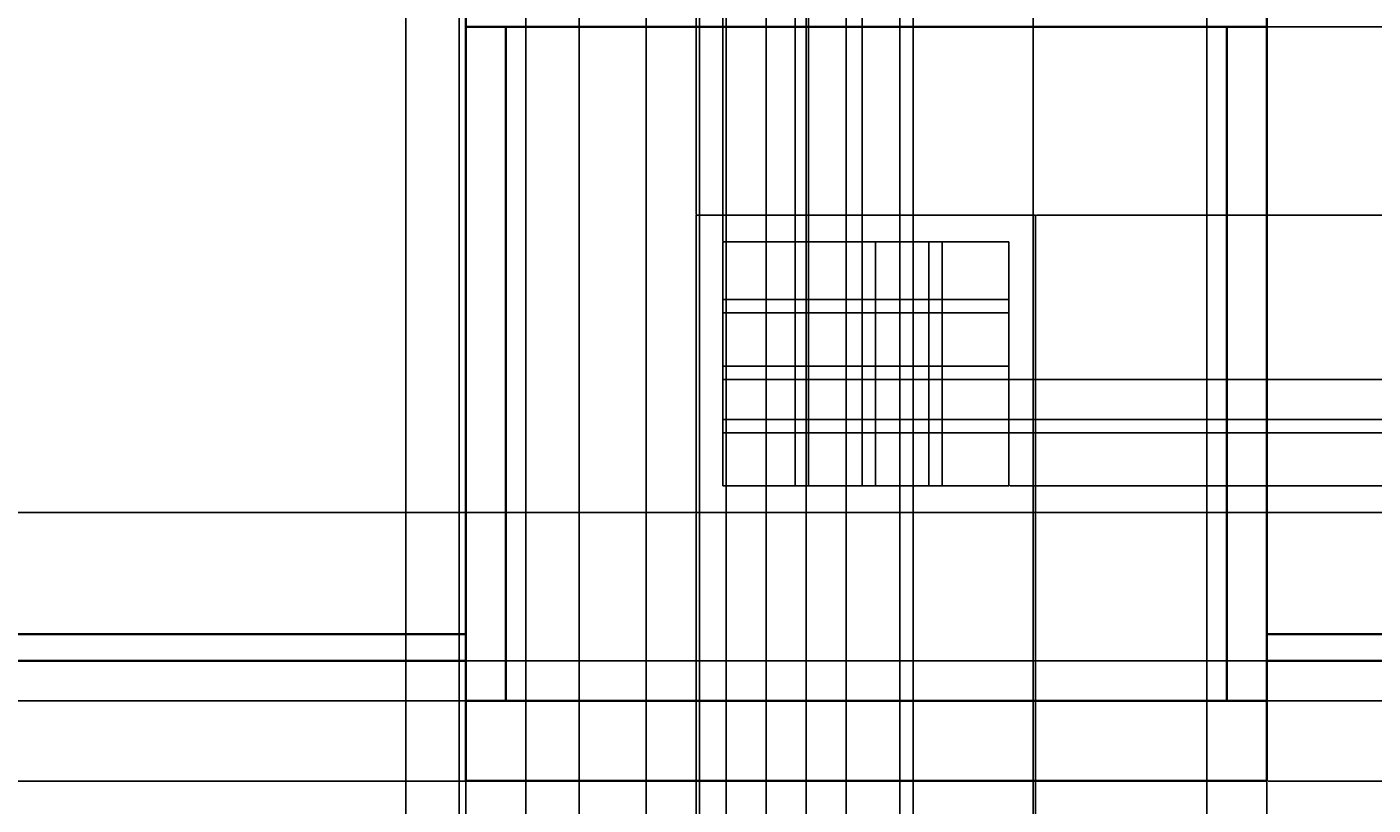
# Model space of a CAD drawing. Units: inches. Extents: x 2154 to 2740, y 571 to 1084.
# Tile 10 of 13: x 2384 to 2485, y 969 to 1027. Entities that reach past the tile are written whole.
import ezdxf

# ---------------------------------------------------------------- set-up
doc = ezdxf.new("R2010")
doc.units = ezdxf.units.IN
for name, color, linetype, lineweight in [('A-ANNO-DIMS', 2, 'Continuous', 18), ('A-GLAZ', 4, 'Continuous', 25), ('A-ROOF', 1, 'Continuous', 35)]:
    doc.layers.add(name, color=color, linetype=linetype, lineweight=lineweight)
doc.styles.get("Standard").update_dxf_attribs({"font": 'arial.ttf'})
doc.dimstyles.get("Standard").update_dxf_attribs({"dimtxt": 0.18, "dimasz": 0.18, "dimexe": 0.18, "dimexo": 0.0625, "dimgap": 0.09, "dimtad": 0, "dimtih": 1, "dimtoh": 1, "dimdec": 4, "dimzin": 0, "dimdsep": 46, "dimtxsty": 'Standard', "dimcen": 0.09, "dimadec": 0, "dimazin": 0, "dimtfac": 1, "dimtdec": 4, "dimtofl": 0, "dimtmove": 0, "dimatfit": 3, "dimfxl": 1, "dimtolj": 1, "dimtzin": 0, "dimarcsym": 0})

# ---------------------------------------------------------------- blocks, each defined once
blk = doc.blocks.new('*D7')
at = {"layer": 'A-ANNO-DIMS', "color": 0, "lineweight": -2, "transparency": 16777216}
for p, q in [((2181.21, 981.59), (2181.21, 1084.04)), ((2181.39, 1083.86), (2446.92, 1083.86)), ((2713.03, 1083.86), (2447.49, 1083.86)), ((2713.21, 981.59), (2713.21, 1084.04))]:
    blk.add_line(p, q, dxfattribs=at)
at = {"layer": 'A-ANNO-DIMS', "color": 0, "transparency": 16777216}
for points in [[(2181.39, 1083.89), (2181.39, 1083.83), (2181.21, 1083.86)], [(2713.03, 1083.89), (2713.03, 1083.83), (2713.21, 1083.86)]]:
    blk.add_solid(points, dxfattribs=at)
at = {"layer": 'Defpoints', "color": 0, "transparency": 16777216}
for p in [(2713.21, 1083.86), (2181.21, 981.53), (2713.21, 981.53)]:
    blk.add_point(p, dxfattribs=at)
at = {"layer": 'A-ANNO-DIMS', "color": 0, "transparency": 16777216, "insert": (2447.21, 1083.86), "char_height": 0.18, "attachment_point": 5}
blk.add_mtext('\\A1;532', dxfattribs=at)
blk = doc.blocks.new('*D9')
at = {"layer": 'A-ANNO-DIMS', "color": 0, "lineweight": -2, "transparency": 16777216}
for p, q in [((2417.21, 970.47), (2417.21, 570.5)), ((2477.21, 970.47), (2477.21, 570.5)), ((2417.39, 570.68), (2446.99, 570.68)), ((2477.03, 570.68), (2447.43, 570.68))]:
    blk.add_line(p, q, dxfattribs=at)
at = {"layer": 'A-ANNO-DIMS', "color": 0, "transparency": 16777216}
for points in [[(2417.39, 570.71), (2417.39, 570.65), (2417.21, 570.68)], [(2477.03, 570.71), (2477.03, 570.65), (2477.21, 570.68)]]:
    blk.add_solid(points, dxfattribs=at)
at = {"layer": 'Defpoints', "color": 0, "transparency": 16777216}
for p in [(2417.21, 970.53), (2477.21, 970.53), (2477.21, 570.68)]:
    blk.add_point(p, dxfattribs=at)
at = {"layer": 'A-ANNO-DIMS', "color": 0, "transparency": 16777216, "insert": (2447.21, 570.68), "char_height": 0.18, "attachment_point": 5}
blk.add_mtext('\\A1;60', dxfattribs=at)
blk = doc.blocks.new('*D10')
at = {"layer": 'A-ANNO-DIMS', "color": 0, "lineweight": -2, "transparency": 16777216}
for p, q in [((2447.14, 1057.01), (2154.18, 1057.01)), ((2154.36, 1056.83), (2154.36, 827.45)), ((2154.36, 597.71), (2154.36, 827.09)), ((2181.14, 597.53), (2154.18, 597.53))]:
    blk.add_line(p, q, dxfattribs=at)
at = {"layer": 'A-ANNO-DIMS', "color": 0, "transparency": 16777216}
for points in [[(2154.33, 1056.83), (2154.39, 1056.83), (2154.36, 1057.01)], [(2154.33, 597.71), (2154.39, 597.71), (2154.36, 597.53)]]:
    blk.add_solid(points, dxfattribs=at)
at = {"layer": 'Defpoints', "color": 0, "transparency": 16777216}
for p in [(2154.36, 1057.01), (2447.21, 1057.01), (2181.21, 597.53)]:
    blk.add_point(p, dxfattribs=at)
at = {"layer": 'A-ANNO-DIMS', "color": 0, "transparency": 16777216, "insert": (2154.36, 827.27), "char_height": 0.18, "attachment_point": 5}
blk.add_mtext('\\A1;459.5', dxfattribs=at)
blk = doc.blocks.new('*D13')
at = {"layer": 'A-ANNO-DIMS', "color": 0, "lineweight": -2, "transparency": 16777216}
for p, q in [((2447.27, 1057.01), (2740.24, 1057.01)), ((2740.06, 1056.83), (2740.06, 1019.45)), ((2740.06, 981.71), (2740.06, 1019.09)), ((2713.27, 981.53), (2740.24, 981.53))]:
    blk.add_line(p, q, dxfattribs=at)
at = {"layer": 'A-ANNO-DIMS', "color": 0, "transparency": 16777216}
for points in [[(2740.03, 1056.83), (2740.09, 1056.83), (2740.06, 1057.01)], [(2740.03, 981.71), (2740.09, 981.71), (2740.06, 981.53)]]:
    blk.add_solid(points, dxfattribs=at)
at = {"layer": 'Defpoints', "color": 0, "transparency": 16777216}
for p in [(2447.21, 1057.01), (2740.06, 1057.01), (2713.21, 981.53)]:
    blk.add_point(p, dxfattribs=at)
at = {"layer": 'A-ANNO-DIMS', "color": 0, "transparency": 16777216, "insert": (2740.06, 1019.27), "char_height": 0.18, "attachment_point": 5}
blk.add_mtext('\\A1;75.47', dxfattribs=at)
blk = doc.blocks.new('*D32')
at = {"layer": 'A-ANNO-DIMS', "color": 0, "lineweight": -2, "transparency": 16777216}
for p, q in [((2412.71, 873.59), (2412.71, 1084.04)), ((2412.89, 1083.86), (2442.49, 1083.86)), ((2472.53, 1083.86), (2442.93, 1083.86)), ((2472.71, 873.59), (2472.71, 1084.04))]:
    blk.add_line(p, q, dxfattribs=at)
at = {"layer": 'A-ANNO-DIMS', "color": 0, "transparency": 16777216}
for points in [[(2412.89, 1083.89), (2412.89, 1083.83), (2412.71, 1083.86)], [(2472.53, 1083.89), (2472.53, 1083.83), (2472.71, 1083.86)]]:
    blk.add_solid(points, dxfattribs=at)
at = {"layer": 'Defpoints', "color": 0, "transparency": 16777216}
for p in [(2472.71, 1083.86), (2412.71, 873.53), (2472.71, 873.53)]:
    blk.add_point(p, dxfattribs=at)
at = {"layer": 'A-ANNO-DIMS', "color": 0, "transparency": 16777216, "insert": (2442.71, 1083.86), "char_height": 0.18, "attachment_point": 5}
blk.add_mtext('\\A1;60', dxfattribs=at)
blk = doc.blocks.new('*D34')
at = {"layer": 'A-ANNO-DIMS', "color": 0, "lineweight": -2, "transparency": 16777216}
for p, q in [((2417.14, 1033.01), (2154.18, 1033.01)), ((2154.36, 1032.83), (2154.36, 1001.96)), ((2154.36, 970.71), (2154.36, 1001.59)), ((2417.14, 970.53), (2154.18, 970.53))]:
    blk.add_line(p, q, dxfattribs=at)
at = {"layer": 'A-ANNO-DIMS', "color": 0, "transparency": 16777216}
for points in [[(2154.33, 1032.83), (2154.39, 1032.83), (2154.36, 1033.01)], [(2154.33, 970.71), (2154.39, 970.71), (2154.36, 970.53)]]:
    blk.add_solid(points, dxfattribs=at)
at = {"layer": 'Defpoints', "color": 0, "transparency": 16777216}
for p in [(2154.36, 1033.01), (2417.21, 1033.01), (2417.21, 970.53)]:
    blk.add_point(p, dxfattribs=at)
at = {"layer": 'A-ANNO-DIMS', "color": 0, "transparency": 16777216, "insert": (2154.36, 1001.77), "char_height": 0.18, "attachment_point": 5}
blk.add_mtext('\\A1;62.48', dxfattribs=at)
blk = doc.blocks.new('*D39')
at = {"layer": 'A-ANNO-DIMS', "color": 0, "lineweight": -2, "transparency": 16777216}
for p, q in [((2183.21, 979.47), (2183.21, 570.5)), ((2417.21, 970.47), (2417.21, 570.5)), ((2183.39, 570.68), (2299.92, 570.68)), ((2417.03, 570.68), (2300.5, 570.68))]:
    blk.add_line(p, q, dxfattribs=at)
at = {"layer": 'A-ANNO-DIMS', "color": 0, "transparency": 16777216}
for points in [[(2183.39, 570.71), (2183.39, 570.65), (2183.21, 570.68)], [(2417.03, 570.71), (2417.03, 570.65), (2417.21, 570.68)]]:
    blk.add_solid(points, dxfattribs=at)
at = {"layer": 'Defpoints', "color": 0, "transparency": 16777216}
for p in [(2183.21, 979.53), (2417.21, 970.53), (2417.21, 570.68)]:
    blk.add_point(p, dxfattribs=at)
at = {"layer": 'A-ANNO-DIMS', "color": 0, "transparency": 16777216, "insert": (2300.21, 570.68), "char_height": 0.18, "attachment_point": 5}
blk.add_mtext('\\A1;234', dxfattribs=at)
blk = doc.blocks.new('*D48')
at = {"layer": 'A-ANNO-DIMS', "color": 0, "lineweight": -2, "transparency": 16777216}
for p, q in [((2195.27, 979.53), (2740.24, 979.53)), ((2740.06, 979.35), (2740.06, 949.71)), ((2740.06, 919.71), (2740.06, 949.35)), ((2195.27, 919.53), (2740.24, 919.53))]:
    blk.add_line(p, q, dxfattribs=at)
at = {"layer": 'A-ANNO-DIMS', "color": 0, "transparency": 16777216}
for points in [[(2740.03, 979.35), (2740.09, 979.35), (2740.06, 979.53)], [(2740.03, 919.71), (2740.09, 919.71), (2740.06, 919.53)]]:
    blk.add_solid(points, dxfattribs=at)
at = {"layer": 'Defpoints', "color": 0, "transparency": 16777216}
for p in [(2195.21, 979.53), (2740.06, 979.53), (2195.21, 919.53)]:
    blk.add_point(p, dxfattribs=at)
at = {"layer": 'A-ANNO-DIMS', "color": 0, "transparency": 16777216, "insert": (2740.06, 949.53), "char_height": 0.18, "attachment_point": 5}
blk.add_mtext('\\A1;60', dxfattribs=at)
blk = doc.blocks.new('*D72')
at = {"layer": 'A-ANNO-DIMS', "color": 0, "lineweight": -2, "transparency": 16777216}
for p, q in [((2477.27, 1027.01), (2740.24, 1027.01)), ((2740.06, 1026.83), (2740.06, 1001.96)), ((2740.06, 976.71), (2740.06, 1001.59)), ((2477.27, 976.53), (2740.24, 976.53))]:
    blk.add_line(p, q, dxfattribs=at)
at = {"layer": 'A-ANNO-DIMS', "color": 0, "transparency": 16777216}
for points in [[(2740.03, 1026.83), (2740.09, 1026.83), (2740.06, 1027.01)], [(2740.03, 976.71), (2740.09, 976.71), (2740.06, 976.53)]]:
    blk.add_solid(points, dxfattribs=at)
at = {"layer": 'Defpoints', "color": 0, "transparency": 16777216}
for p in [(2477.21, 1027.01), (2740.06, 1027.01), (2477.21, 976.53)]:
    blk.add_point(p, dxfattribs=at)
at = {"layer": 'A-ANNO-DIMS', "color": 0, "transparency": 16777216, "insert": (2740.06, 1001.77), "char_height": 0.18, "attachment_point": 5}
blk.add_mtext('\\A1;50.48', dxfattribs=at)
blk = doc.blocks.new('*D73')
at = {"layer": 'A-ANNO-DIMS', "color": 0, "lineweight": -2, "transparency": 16777216}
for p, q in [((2477.27, 976.53), (2740.24, 976.53)), ((2740.06, 976.35), (2740.06, 973.71)), ((2740.06, 970.71), (2740.06, 973.35)), ((2477.27, 970.53), (2740.24, 970.53))]:
    blk.add_line(p, q, dxfattribs=at)
at = {"layer": 'A-ANNO-DIMS', "color": 0, "transparency": 16777216}
for points in [[(2740.03, 976.35), (2740.09, 976.35), (2740.06, 976.53)], [(2740.03, 970.71), (2740.09, 970.71), (2740.06, 970.53)]]:
    blk.add_solid(points, dxfattribs=at)
at = {"layer": 'Defpoints', "color": 0, "transparency": 16777216}
for p in [(2477.21, 976.53), (2740.06, 976.53), (2477.21, 970.53)]:
    blk.add_point(p, dxfattribs=at)
at = {"layer": 'A-ANNO-DIMS', "color": 0, "transparency": 16777216, "insert": (2740.06, 973.53), "char_height": 0.18, "attachment_point": 5}
blk.add_mtext('\\A1;6', dxfattribs=at)
blk = doc.blocks.new('*D75')
at = {"layer": 'A-ANNO-DIMS', "color": 0, "lineweight": -2, "transparency": 16777216}
for p, q in [((2434.46, 990.57), (2434.46, 570.5)), ((2417.21, 981.47), (2417.21, 570.5)), ((2417.39, 570.68), (2425.45, 570.68)), ((2434.28, 570.68), (2426.22, 570.68))]:
    blk.add_line(p, q, dxfattribs=at)
at = {"layer": 'A-ANNO-DIMS', "color": 0, "transparency": 16777216}
for points in [[(2417.39, 570.71), (2417.39, 570.65), (2417.21, 570.68)], [(2434.28, 570.71), (2434.28, 570.65), (2434.46, 570.68)]]:
    blk.add_solid(points, dxfattribs=at)
at = {"layer": 'Defpoints', "color": 0, "transparency": 16777216}
for p in [(2434.46, 990.64), (2417.21, 981.53), (2434.46, 570.68)]:
    blk.add_point(p, dxfattribs=at)
at = {"layer": 'A-ANNO-DIMS', "color": 0, "transparency": 16777216, "insert": (2425.83, 570.68), "char_height": 0.18, "attachment_point": 5}
blk.add_mtext('\\A1;17.25', dxfattribs=at)
blk = doc.blocks.new('*D76')
at = {"layer": 'A-ANNO-DIMS', "color": 0, "lineweight": -2, "transparency": 16777216}
for p, q in [((2434.46, 990.57), (2434.46, 570.5)), ((2459.89, 990.57), (2459.89, 570.5)), ((2434.64, 570.68), (2446.71, 570.68)), ((2459.71, 570.68), (2447.64, 570.68))]:
    blk.add_line(p, q, dxfattribs=at)
at = {"layer": 'A-ANNO-DIMS', "color": 0, "transparency": 16777216}
for points in [[(2434.64, 570.71), (2434.64, 570.65), (2434.46, 570.68)], [(2459.71, 570.71), (2459.71, 570.65), (2459.89, 570.68)]]:
    blk.add_solid(points, dxfattribs=at)
at = {"layer": 'Defpoints', "color": 0, "transparency": 16777216}
for p in [(2434.46, 990.64), (2459.89, 990.64), (2459.89, 570.68)]:
    blk.add_point(p, dxfattribs=at)
at = {"layer": 'A-ANNO-DIMS', "color": 0, "transparency": 16777216, "insert": (2447.17, 570.68), "char_height": 0.18, "attachment_point": 5}
blk.add_mtext('\\A1;25.433', dxfattribs=at)
blk = doc.blocks.new('*D77')
at = {"layer": 'A-ANNO-DIMS', "color": 0, "lineweight": -2, "transparency": 16777216}
for p, q in [((2434.39, 990.64), (2154.18, 990.64)), ((2154.36, 990.46), (2154.36, 983.77)), ((2154.36, 976.71), (2154.36, 983.4)), ((2420.14, 976.53), (2154.18, 976.53))]:
    blk.add_line(p, q, dxfattribs=at)
at = {"layer": 'A-ANNO-DIMS', "color": 0, "transparency": 16777216}
for points in [[(2154.33, 990.46), (2154.39, 990.46), (2154.36, 990.64)], [(2154.33, 976.71), (2154.39, 976.71), (2154.36, 976.53)]]:
    blk.add_solid(points, dxfattribs=at)
at = {"layer": 'Defpoints', "color": 0, "transparency": 16777216}
for p in [(2154.36, 990.64), (2434.46, 990.64), (2420.21, 976.53)]:
    blk.add_point(p, dxfattribs=at)
at = {"layer": 'A-ANNO-DIMS', "color": 0, "transparency": 16777216, "insert": (2154.36, 983.58), "char_height": 0.18, "attachment_point": 5}
blk.add_mtext('\\A1;14.104', dxfattribs=at)
blk = doc.blocks.new('*D78')
at = {"layer": 'A-ANNO-DIMS', "color": 0, "lineweight": -2, "transparency": 16777216}
for p, q in [((2459.95, 1012.91), (2740.24, 1012.91)), ((2740.06, 1012.73), (2740.06, 1001.95)), ((2740.06, 990.82), (2740.06, 1001.59)), ((2459.95, 990.64), (2740.24, 990.64))]:
    blk.add_line(p, q, dxfattribs=at)
at = {"layer": 'A-ANNO-DIMS', "color": 0, "transparency": 16777216}
for points in [[(2740.03, 1012.73), (2740.09, 1012.73), (2740.06, 1012.91)], [(2740.03, 990.82), (2740.09, 990.82), (2740.06, 990.64)]]:
    blk.add_solid(points, dxfattribs=at)
at = {"layer": 'Defpoints', "color": 0, "transparency": 16777216}
for p in [(2459.89, 1012.91), (2740.06, 1012.91), (2459.89, 990.64)]:
    blk.add_point(p, dxfattribs=at)
at = {"layer": 'A-ANNO-DIMS', "color": 0, "transparency": 16777216, "insert": (2740.06, 1001.77), "char_height": 0.18, "attachment_point": 5}
blk.add_mtext('\\A1;22.27', dxfattribs=at)
blk = doc.blocks.new('*D79')
at = {"layer": 'A-ANNO-DIMS', "color": 0, "lineweight": -2, "transparency": 16777216}
for p, q in [((2436.46, 1010.97), (2436.46, 1084.04)), ((2436.64, 1083.86), (2438.78, 1083.86)), ((2441.71, 1083.86), (2439.57, 1083.86)), ((2441.89, 1010.97), (2441.89, 1084.04))]:
    blk.add_line(p, q, dxfattribs=at)
at = {"layer": 'A-ANNO-DIMS', "color": 0, "transparency": 16777216}
for points in [[(2436.64, 1083.89), (2436.64, 1083.83), (2436.46, 1083.86)], [(2441.71, 1083.89), (2441.71, 1083.83), (2441.89, 1083.86)]]:
    blk.add_solid(points, dxfattribs=at)
at = {"layer": 'Defpoints', "color": 0, "transparency": 16777216}
for p in [(2441.89, 1083.86), (2436.46, 1010.91), (2441.89, 1010.91)]:
    blk.add_point(p, dxfattribs=at)
at = {"layer": 'A-ANNO-DIMS', "color": 0, "transparency": 16777216, "insert": (2439.17, 1083.86), "char_height": 0.18, "attachment_point": 5}
blk.add_mtext('\\A1;5.433', dxfattribs=at)
blk = doc.blocks.new('*D80')
at = {"layer": 'A-ANNO-DIMS', "color": 0, "lineweight": -2, "transparency": 16777216}
for p, q in [((2441.89, 1010.97), (2441.89, 1084.04)), ((2442.07, 1083.86), (2442.27, 1083.86)), ((2442.71, 1083.86), (2442.51, 1083.86)), ((2442.89, 1010.97), (2442.89, 1084.04))]:
    blk.add_line(p, q, dxfattribs=at)
at = {"layer": 'A-ANNO-DIMS', "color": 0, "transparency": 16777216}
for points in [[(2442.07, 1083.89), (2442.07, 1083.83), (2441.89, 1083.86)], [(2442.71, 1083.89), (2442.71, 1083.83), (2442.89, 1083.86)]]:
    blk.add_solid(points, dxfattribs=at)
at = {"layer": 'Defpoints', "color": 0, "transparency": 16777216}
for p in [(2442.89, 1083.86), (2441.89, 1010.91), (2442.89, 1010.91)]:
    blk.add_point(p, dxfattribs=at)
at = {"layer": 'A-ANNO-DIMS', "color": 0, "transparency": 16777216, "insert": (2442.39, 1083.86), "char_height": 0.18, "attachment_point": 5}
blk.add_mtext('\\A1;1', dxfattribs=at)
blk = doc.blocks.new('*D81')
at = {"layer": 'A-ANNO-DIMS', "color": 0, "lineweight": -2, "transparency": 16777216}
for p, q in [((2442.89, 1010.97), (2442.89, 1084.04)), ((2443.07, 1083.86), (2444.74, 1083.86)), ((2446.71, 1083.86), (2445.04, 1083.86)), ((2446.89, 1010.97), (2446.89, 1084.04))]:
    blk.add_line(p, q, dxfattribs=at)
at = {"layer": 'A-ANNO-DIMS', "color": 0, "transparency": 16777216}
for points in [[(2443.07, 1083.89), (2443.07, 1083.83), (2442.89, 1083.86)], [(2446.71, 1083.89), (2446.71, 1083.83), (2446.89, 1083.86)]]:
    blk.add_solid(points, dxfattribs=at)
at = {"layer": 'Defpoints', "color": 0, "transparency": 16777216}
for p in [(2446.89, 1083.86), (2442.89, 1010.91), (2446.89, 1010.91)]:
    blk.add_point(p, dxfattribs=at)
at = {"layer": 'A-ANNO-DIMS', "color": 0, "transparency": 16777216, "insert": (2444.89, 1083.86), "char_height": 0.18, "attachment_point": 5}
blk.add_mtext('\\A1;4', dxfattribs=at)
blk = doc.blocks.new('*D82')
at = {"layer": 'A-ANNO-DIMS', "color": 0, "lineweight": -2, "transparency": 16777216}
for p, q in [((2434.46, 1012.97), (2434.46, 1084.04)), ((2434.64, 1083.86), (2435.31, 1083.86)), ((2436.28, 1083.86), (2435.61, 1083.86)), ((2436.46, 1010.97), (2436.46, 1084.04))]:
    blk.add_line(p, q, dxfattribs=at)
at = {"layer": 'A-ANNO-DIMS', "color": 0, "transparency": 16777216}
for points in [[(2434.64, 1083.89), (2434.64, 1083.83), (2434.46, 1083.86)], [(2436.28, 1083.89), (2436.28, 1083.83), (2436.46, 1083.86)]]:
    blk.add_solid(points, dxfattribs=at)
at = {"layer": 'Defpoints', "color": 0, "transparency": 16777216}
for p in [(2436.46, 1083.86), (2434.46, 1012.91), (2436.46, 1010.91)]:
    blk.add_point(p, dxfattribs=at)
at = {"layer": 'A-ANNO-DIMS', "color": 0, "transparency": 16777216, "insert": (2435.46, 1083.86), "char_height": 0.18, "attachment_point": 5}
blk.add_mtext('\\A1;2', dxfattribs=at)
blk = doc.blocks.new('*D83')
at = {"layer": 'A-ANNO-DIMS', "color": 0, "lineweight": -2, "transparency": 16777216}
for p, q in [((2457.95, 996.6), (2740.24, 996.6)), ((2740.06, 996.42), (2740.06, 994.8)), ((2740.06, 992.82), (2740.06, 994.44)), ((2457.95, 992.64), (2740.24, 992.64))]:
    blk.add_line(p, q, dxfattribs=at)
at = {"layer": 'A-ANNO-DIMS', "color": 0, "transparency": 16777216}
for points in [[(2740.03, 996.42), (2740.09, 996.42), (2740.06, 996.6)], [(2740.03, 992.82), (2740.09, 992.82), (2740.06, 992.64)]]:
    blk.add_solid(points, dxfattribs=at)
at = {"layer": 'Defpoints', "color": 0, "transparency": 16777216}
for p in [(2457.89, 996.6), (2740.06, 996.6), (2457.89, 992.64)]:
    blk.add_point(p, dxfattribs=at)
at = {"layer": 'A-ANNO-DIMS', "color": 0, "transparency": 16777216, "insert": (2740.06, 994.62), "char_height": 0.18, "attachment_point": 5}
blk.add_mtext('\\A1;3.964', dxfattribs=at)
blk = doc.blocks.new('*D84')
at = {"layer": 'A-ANNO-DIMS', "color": 0, "lineweight": -2, "transparency": 16777216}
for p, q in [((2457.95, 997.6), (2740.24, 997.6)), ((2740.06, 997.42), (2740.06, 997.28)), ((2457.95, 996.6), (2740.24, 996.6)), ((2740.06, 996.78), (2740.06, 996.92))]:
    blk.add_line(p, q, dxfattribs=at)
at = {"layer": 'A-ANNO-DIMS', "color": 0, "transparency": 16777216}
for points in [[(2740.03, 997.42), (2740.09, 997.42), (2740.06, 997.6)], [(2740.03, 996.78), (2740.09, 996.78), (2740.06, 996.6)]]:
    blk.add_solid(points, dxfattribs=at)
at = {"layer": 'Defpoints', "color": 0, "transparency": 16777216}
for p in [(2457.89, 997.6), (2740.06, 997.6), (2457.89, 996.6)]:
    blk.add_point(p, dxfattribs=at)
at = {"layer": 'A-ANNO-DIMS', "color": 0, "transparency": 16777216, "insert": (2740.06, 997.1), "char_height": 0.18, "attachment_point": 5}
blk.add_mtext('\\A1;1', dxfattribs=at)
blk = doc.blocks.new('*D85')
at = {"layer": 'A-ANNO-DIMS', "color": 0, "lineweight": -2, "transparency": 16777216}
for p, q in [((2457.95, 1000.6), (2740.24, 1000.6)), ((2740.06, 1000.42), (2740.06, 999.28)), ((2740.06, 997.78), (2740.06, 998.92)), ((2457.95, 997.6), (2740.24, 997.6))]:
    blk.add_line(p, q, dxfattribs=at)
at = {"layer": 'A-ANNO-DIMS', "color": 0, "transparency": 16777216}
for points in [[(2740.03, 1000.42), (2740.09, 1000.42), (2740.06, 1000.6)], [(2740.03, 997.78), (2740.09, 997.78), (2740.06, 997.6)]]:
    blk.add_solid(points, dxfattribs=at)
at = {"layer": 'Defpoints', "color": 0, "transparency": 16777216}
for p in [(2457.89, 1000.6), (2740.06, 1000.6), (2457.89, 997.6)]:
    blk.add_point(p, dxfattribs=at)
at = {"layer": 'A-ANNO-DIMS', "color": 0, "transparency": 16777216, "insert": (2740.06, 999.1), "char_height": 0.18, "attachment_point": 5}
blk.add_mtext('\\A1;3', dxfattribs=at)
blk = doc.blocks.new('*D87')
at = {"layer": 'A-ANNO-DIMS', "color": 0, "lineweight": -2, "transparency": 16777216}
for p, q in [((2421.71, 725.29), (2421.71, 1084.04)), ((2421.89, 1083.86), (2423.55, 1083.86)), ((2425.53, 1083.86), (2423.86, 1083.86)), ((2425.71, 721.29), (2425.71, 1084.04))]:
    blk.add_line(p, q, dxfattribs=at)
at = {"layer": 'A-ANNO-DIMS', "color": 0, "transparency": 16777216}
for points in [[(2421.89, 1083.89), (2421.89, 1083.83), (2421.71, 1083.86)], [(2425.53, 1083.89), (2425.53, 1083.83), (2425.71, 1083.86)]]:
    blk.add_solid(points, dxfattribs=at)
at = {"layer": 'Defpoints', "color": 0, "transparency": 16777216}
for p in [(2425.71, 1083.86), (2421.71, 725.23), (2425.71, 721.23)]:
    blk.add_point(p, dxfattribs=at)
at = {"layer": 'A-ANNO-DIMS', "color": 0, "transparency": 16777216, "insert": (2423.71, 1083.86), "char_height": 0.18, "attachment_point": 5}
blk.add_mtext('\\A1;4', dxfattribs=at)
blk = doc.blocks.new('*D90')
at = {"layer": 'A-ANNO-DIMS', "color": 0, "lineweight": -2, "transparency": 16777216}
for p, q in [((2434.71, 712.29), (2434.71, 1084.04)), ((2434.89, 1083.86), (2442.5, 1083.86)), ((2450.53, 1083.86), (2442.92, 1083.86)), ((2450.71, 712.29), (2450.71, 1084.04))]:
    blk.add_line(p, q, dxfattribs=at)
at = {"layer": 'A-ANNO-DIMS', "color": 0, "transparency": 16777216}
for points in [[(2434.89, 1083.89), (2434.89, 1083.83), (2434.71, 1083.86)], [(2450.53, 1083.89), (2450.53, 1083.83), (2450.71, 1083.86)]]:
    blk.add_solid(points, dxfattribs=at)
at = {"layer": 'Defpoints', "color": 0, "transparency": 16777216}
for p in [(2450.71, 1083.86), (2434.71, 712.23), (2450.71, 712.23)]:
    blk.add_point(p, dxfattribs=at)
at = {"layer": 'A-ANNO-DIMS', "color": 0, "transparency": 16777216, "insert": (2442.71, 1083.86), "char_height": 0.18, "attachment_point": 5}
blk.add_mtext('\\A1;16', dxfattribs=at)
blk = doc.blocks.new('*D93')
at = {"layer": 'A-ANNO-DIMS', "color": 0, "lineweight": -2, "transparency": 16777216}
for p, q in [((2439.71, 703.29), (2439.71, 1084.04)), ((2439.89, 1083.86), (2442.56, 1083.86)), ((2445.53, 1083.86), (2442.86, 1083.86)), ((2445.71, 703.29), (2445.71, 1084.04))]:
    blk.add_line(p, q, dxfattribs=at)
at = {"layer": 'A-ANNO-DIMS', "color": 0, "transparency": 16777216}
for points in [[(2439.89, 1083.89), (2439.89, 1083.83), (2439.71, 1083.86)], [(2445.53, 1083.89), (2445.53, 1083.83), (2445.71, 1083.86)]]:
    blk.add_solid(points, dxfattribs=at)
at = {"layer": 'Defpoints', "color": 0, "transparency": 16777216}
for p in [(2445.71, 1083.86), (2439.71, 703.23), (2445.71, 703.23)]:
    blk.add_point(p, dxfattribs=at)
at = {"layer": 'A-ANNO-DIMS', "color": 0, "transparency": 16777216, "insert": (2442.71, 1083.86), "char_height": 0.18, "attachment_point": 5}
blk.add_mtext('\\A1;6', dxfattribs=at)
blk = doc.blocks.new('*D94')
at = {"layer": 'A-ANNO-DIMS', "color": 0, "lineweight": -2, "transparency": 16777216}
for p, q in [((2445.71, 703.29), (2445.71, 1084.04)), ((2445.89, 1083.86), (2447.55, 1083.86)), ((2449.53, 1083.86), (2447.86, 1083.86)), ((2449.71, 703.29), (2449.71, 1084.04))]:
    blk.add_line(p, q, dxfattribs=at)
at = {"layer": 'A-ANNO-DIMS', "color": 0, "transparency": 16777216}
for points in [[(2445.89, 1083.89), (2445.89, 1083.83), (2445.71, 1083.86)], [(2449.53, 1083.89), (2449.53, 1083.83), (2449.71, 1083.86)]]:
    blk.add_solid(points, dxfattribs=at)
at = {"layer": 'Defpoints', "color": 0, "transparency": 16777216}
for p in [(2449.71, 1083.86), (2445.71, 703.23), (2449.71, 703.23)]:
    blk.add_point(p, dxfattribs=at)
at = {"layer": 'A-ANNO-DIMS', "color": 0, "transparency": 16777216, "insert": (2447.71, 1083.86), "char_height": 0.18, "attachment_point": 5}
blk.add_mtext('\\A1;4', dxfattribs=at)
blk = doc.blocks.new('*D99')
at = {"layer": 'A-ANNO-DIMS', "color": 0, "lineweight": -2, "transparency": 16777216}
for p, q in [((2412.71, 873.59), (2412.71, 1084.04)), ((2412.89, 1083.86), (2414.55, 1083.86)), ((2416.53, 1083.86), (2414.86, 1083.86)), ((2416.71, 869.59), (2416.71, 1084.04))]:
    blk.add_line(p, q, dxfattribs=at)
at = {"layer": 'A-ANNO-DIMS', "color": 0, "transparency": 16777216}
for points in [[(2412.89, 1083.89), (2412.89, 1083.83), (2412.71, 1083.86)], [(2416.53, 1083.89), (2416.53, 1083.83), (2416.71, 1083.86)]]:
    blk.add_solid(points, dxfattribs=at)
at = {"layer": 'Defpoints', "color": 0, "transparency": 16777216}
for p in [(2416.71, 1083.86), (2412.71, 873.53), (2416.71, 869.53)]:
    blk.add_point(p, dxfattribs=at)
at = {"layer": 'A-ANNO-DIMS', "color": 0, "transparency": 16777216, "insert": (2414.71, 1083.86), "char_height": 0.18, "attachment_point": 5}
blk.add_mtext('\\A1;4', dxfattribs=at)
blk = doc.blocks.new('*D101')
at = {"layer": 'A-ANNO-DIMS', "color": 0, "lineweight": -2, "transparency": 16777216}
for p, q in [((2416.71, 869.59), (2416.71, 1084.04)), ((2416.89, 1083.86), (2421.06, 1083.86)), ((2425.53, 1083.86), (2421.36, 1083.86)), ((2425.71, 860.59), (2425.71, 1084.04))]:
    blk.add_line(p, q, dxfattribs=at)
at = {"layer": 'A-ANNO-DIMS', "color": 0, "transparency": 16777216}
for points in [[(2416.89, 1083.89), (2416.89, 1083.83), (2416.71, 1083.86)], [(2425.53, 1083.89), (2425.53, 1083.83), (2425.71, 1083.86)]]:
    blk.add_solid(points, dxfattribs=at)
at = {"layer": 'Defpoints', "color": 0, "transparency": 16777216}
for p in [(2425.71, 1083.86), (2416.71, 869.53), (2425.71, 860.53)]:
    blk.add_point(p, dxfattribs=at)
at = {"layer": 'A-ANNO-DIMS', "color": 0, "transparency": 16777216, "insert": (2421.21, 1083.86), "char_height": 0.18, "attachment_point": 5}
blk.add_mtext('\\A1;9', dxfattribs=at)
blk = doc.blocks.new('*D102')
at = {"layer": 'A-ANNO-DIMS', "color": 0, "lineweight": -2, "transparency": 16777216}
for p, q in [((2425.71, 860.59), (2425.71, 1084.04)), ((2425.89, 1083.86), (2428.06, 1083.86)), ((2430.53, 1083.86), (2428.36, 1083.86)), ((2430.71, 860.59), (2430.71, 1084.04))]:
    blk.add_line(p, q, dxfattribs=at)
at = {"layer": 'A-ANNO-DIMS', "color": 0, "transparency": 16777216}
for points in [[(2425.89, 1083.89), (2425.89, 1083.83), (2425.71, 1083.86)], [(2430.53, 1083.89), (2430.53, 1083.83), (2430.71, 1083.86)]]:
    blk.add_solid(points, dxfattribs=at)
at = {"layer": 'Defpoints', "color": 0, "transparency": 16777216}
for p in [(2430.71, 1083.86), (2425.71, 860.53), (2430.71, 860.53)]:
    blk.add_point(p, dxfattribs=at)
at = {"layer": 'A-ANNO-DIMS', "color": 0, "transparency": 16777216, "insert": (2428.21, 1083.86), "char_height": 0.18, "attachment_point": 5}
blk.add_mtext('\\A1;5', dxfattribs=at)
blk = doc.blocks.new('*D103')
at = {"layer": 'A-ANNO-DIMS', "color": 0, "lineweight": -2, "transparency": 16777216}
for p, q in [((2430.71, 860.59), (2430.71, 1084.04)), ((2430.89, 1083.86), (2433.56, 1083.86)), ((2436.53, 1083.86), (2433.86, 1083.86)), ((2436.71, 860.59), (2436.71, 1084.04))]:
    blk.add_line(p, q, dxfattribs=at)
at = {"layer": 'A-ANNO-DIMS', "color": 0, "transparency": 16777216}
for points in [[(2430.89, 1083.89), (2430.89, 1083.83), (2430.71, 1083.86)], [(2436.53, 1083.89), (2436.53, 1083.83), (2436.71, 1083.86)]]:
    blk.add_solid(points, dxfattribs=at)
at = {"layer": 'Defpoints', "color": 0, "transparency": 16777216}
for p in [(2436.71, 1083.86), (2430.71, 860.53), (2436.71, 860.53)]:
    blk.add_point(p, dxfattribs=at)
at = {"layer": 'A-ANNO-DIMS', "color": 0, "transparency": 16777216, "insert": (2433.71, 1083.86), "char_height": 0.18, "attachment_point": 5}
blk.add_mtext('\\A1;6', dxfattribs=at)
blk = doc.blocks.new('*D104')
at = {"layer": 'A-ANNO-DIMS', "color": 0, "lineweight": -2, "transparency": 16777216}
for p, q in [((2436.71, 860.59), (2436.71, 1084.04)), ((2436.89, 1083.86), (2439.56, 1083.86)), ((2442.53, 1083.86), (2439.86, 1083.86)), ((2442.71, 860.59), (2442.71, 1084.04))]:
    blk.add_line(p, q, dxfattribs=at)
at = {"layer": 'A-ANNO-DIMS', "color": 0, "transparency": 16777216}
for points in [[(2436.89, 1083.89), (2436.89, 1083.83), (2436.71, 1083.86)], [(2442.53, 1083.89), (2442.53, 1083.83), (2442.71, 1083.86)]]:
    blk.add_solid(points, dxfattribs=at)
at = {"layer": 'Defpoints', "color": 0, "transparency": 16777216}
for p in [(2442.71, 1083.86), (2436.71, 860.53), (2442.71, 860.53)]:
    blk.add_point(p, dxfattribs=at)
at = {"layer": 'A-ANNO-DIMS', "color": 0, "transparency": 16777216, "insert": (2439.71, 1083.86), "char_height": 0.18, "attachment_point": 5}
blk.add_mtext('\\A1;6', dxfattribs=at)
blk = doc.blocks.new('*D105')
at = {"layer": 'A-ANNO-DIMS', "color": 0, "lineweight": -2, "transparency": 16777216}
for p, q in [((2442.71, 860.59), (2442.71, 1084.04)), ((2442.89, 1083.86), (2451, 1083.86)), ((2459.53, 1083.86), (2451.42, 1083.86)), ((2459.71, 860.59), (2459.71, 1084.04))]:
    blk.add_line(p, q, dxfattribs=at)
at = {"layer": 'A-ANNO-DIMS', "color": 0, "transparency": 16777216}
for points in [[(2442.89, 1083.89), (2442.89, 1083.83), (2442.71, 1083.86)], [(2459.53, 1083.89), (2459.53, 1083.83), (2459.71, 1083.86)]]:
    blk.add_solid(points, dxfattribs=at)
at = {"layer": 'Defpoints', "color": 0, "transparency": 16777216}
for p in [(2459.71, 1083.86), (2442.71, 860.53), (2459.71, 860.53)]:
    blk.add_point(p, dxfattribs=at)
at = {"layer": 'A-ANNO-DIMS', "color": 0, "transparency": 16777216, "insert": (2451.21, 1083.86), "char_height": 0.18, "attachment_point": 5}
blk.add_mtext('\\A1;17', dxfattribs=at)

msp = doc.modelspace()

# ---------------------------------------------------------------- linework, layer by layer
at = {"layer": 'A-GLAZ'}
for p, q in [((2436.4565, 1010.9076), (2457.8896, 1010.9076)), ((2436.4565, 992.6361), (2436.4565, 1010.9076)), ((2441.8896, 1010.9076), (2441.8896, 992.6361)), ((2442.8896, 1010.9076), (2442.8896, 992.6361)), ((2446.8896, 1010.9076), (2446.8896, 992.6361)), ((2447.8896, 1010.9076), (2447.8896, 992.6361)), ((2451.8896, 1010.9076), (2451.8896, 992.6361)), ((2452.8896, 1010.9076), (2452.8896, 992.6361)), ((2457.8896, 1010.9076), (2457.8896, 992.6361)), ((2457.8896, 1006.5998), (2436.4565, 1006.5998)), ((2457.8896, 1005.5998), (2436.4565, 1005.5998)), ((2457.8896, 1001.5998), (2436.4565, 1001.5998)), ((2457.8896, 1000.5998), (2436.4565, 1000.5998)), ((2457.8896, 997.5998), (2436.4565, 997.5998)), ((2457.8896, 996.5998), (2436.4565, 996.5998)), ((2457.8896, 992.6361), (2436.4565, 992.6361))]:
    msp.add_line(p, q, dxfattribs=at)
msp.add_lwpolyline([(2434.4565, 1012.9076), (2459.8896, 1012.9076), (2459.8896, 990.6361), (2434.4565, 990.6361)], close=True, dxfattribs=at)
at = {"layer": 'A-ROOF'}
for p, q in [((2417.2067, 970.5321), (2417.2067, 1035.2521)), ((2477.2067, 970.5321), (2477.2067, 1035.2521)), ((2417.2067, 1027.0148), (2477.2067, 1027.0148)), ((2420.2067, 976.5321), (2420.2067, 1027.0148)), ((2474.2067, 976.5321), (2474.2067, 1027.0148)), ((2181.2067, 981.5321), (2417.2067, 981.5321)), ((2477.2067, 981.5321), (2713.2067, 981.5321)), ((2183.2067, 979.5321), (2417.2067, 979.5321)), ((2477.2067, 979.5321), (2711.2067, 979.5321)), ((2417.2067, 976.5321), (2477.2067, 976.5321)), ((2417.2067, 970.5321), (2477.2067, 970.5321))]:
    msp.add_line(p, q, dxfattribs=at)

# ---------------------------------------------------------------- dimensions: what is measured, and where the dimension line sits
at = {"layer": 'A-ANNO-DIMS'}
for base, p1, p2, override, picture, middle in [((2713.2067, 1083.8553), (2181.2067, 981.5321), (2713.2067, 981.5321), {"dimdec": 0, "dimlfac": 1, "dimrnd": 0, "dimzin": 0, "dimdsep": 46, "dimlunit": 2}, '*D7', (2447.2067, 1083.8553)), ((2472.7067, 1083.8553), (2412.7067, 873.5321), (2472.7067, 873.5321), {"dimdec": 0, "dimlfac": 1, "dimrnd": 0, "dimzin": 0, "dimdsep": 46, "dimlunit": 2}, '*D32', (2442.7067, 1083.8553)), ((2416.7067, 1083.8553), (2412.7067, 873.5321), (2416.7067, 869.5321), {"dimdec": 0, "dimlfac": 1, "dimrnd": 0, "dimzin": 0, "dimdsep": 46, "dimlunit": 2}, '*D99', (2414.7067, 1083.8553)), ((2425.7067, 1083.8553), (2416.7067, 869.5321), (2425.7067, 860.5321), {"dimdec": 0, "dimlfac": 1, "dimrnd": 0, "dimzin": 0, "dimdsep": 46, "dimlunit": 2}, '*D101', (2421.2067, 1083.8553)), ((2425.7067, 1083.8553), (2421.7067, 725.2281), (2425.7067, 721.2281), {"dimdec": 0, "dimlfac": 1, "dimrnd": 0, "dimzin": 0, "dimdsep": 46, "dimlunit": 2}, '*D87', (2423.7067, 1083.8553)), ((2430.7067, 1083.8553), (2425.7067, 860.5321), (2430.7067, 860.5321), {"dimdec": 0, "dimlfac": 1, "dimrnd": 0, "dimzin": 0, "dimdsep": 46, "dimlunit": 2}, '*D102', (2428.2067, 1083.8553)), ((2436.7067, 1083.8553), (2430.7067, 860.5321), (2436.7067, 860.5321), {"dimdec": 0, "dimlfac": 1, "dimrnd": 0, "dimzin": 0, "dimdsep": 46, "dimlunit": 2}, '*D103', (2433.7067, 1083.8553)), ((2436.4565, 1083.8553), (2434.4565, 1012.9076), (2436.4565, 1010.9076), {"dimdec": 0, "dimlfac": 1, "dimrnd": 0, "dimzin": 0, "dimdsep": 46, "dimlunit": 2}, '*D82', (2435.4565, 1083.8553)), ((2450.7067, 1083.8553), (2434.7067, 712.2281), (2450.7067, 712.2281), {"dimdec": 0, "dimlfac": 1, "dimrnd": 0, "dimzin": 0, "dimdsep": 46, "dimlunit": 2}, '*D90', (2442.7067, 1083.8553)), ((2441.8896, 1083.8553), (2436.4565, 1010.9076), (2441.8896, 1010.9076), {"dimdec": 3, "dimlfac": 1, "dimrnd": 0, "dimzin": 0, "dimdsep": 46, "dimlunit": 2}, '*D79', (2439.173, 1083.8553)), ((2442.7067, 1083.8553), (2436.7067, 860.5321), (2442.7067, 860.5321), {"dimdec": 0, "dimlfac": 1, "dimrnd": 0, "dimzin": 0, "dimdsep": 46, "dimlunit": 2}, '*D104', (2439.7067, 1083.8553)), ((2445.7067, 1083.8553), (2439.7067, 703.2281), (2445.7067, 703.2281), {"dimdec": 0, "dimlfac": 1, "dimrnd": 0, "dimzin": 0, "dimdsep": 46, "dimlunit": 2}, '*D93', (2442.7067, 1083.8553)), ((2442.8896, 1083.8553), (2441.8896, 1010.9076), (2442.8896, 1010.9076), {"dimdec": 0, "dimlfac": 1, "dimrnd": 0, "dimzin": 0, "dimdsep": 46, "dimlunit": 2}, '*D80', (2442.3896, 1083.8553)), ((2459.7067, 1083.8553), (2442.7067, 860.5321), (2459.7067, 860.5321), {"dimdec": 0, "dimlfac": 1, "dimrnd": 0, "dimzin": 0, "dimdsep": 46, "dimlunit": 2}, '*D105', (2451.2067, 1083.8553)), ((2446.8896, 1083.8553), (2442.8896, 1010.9076), (2446.8896, 1010.9076), {"dimdec": 0, "dimlfac": 1, "dimrnd": 0, "dimzin": 0, "dimdsep": 46, "dimlunit": 2}, '*D81', (2444.8896, 1083.8553)), ((2449.7067, 1083.8553), (2445.7067, 703.2281), (2449.7067, 703.2281), {"dimdec": 0, "dimlfac": 1, "dimrnd": 0, "dimzin": 0, "dimdsep": 46, "dimlunit": 2}, '*D94', (2447.7067, 1083.8553)), ((2434.4565, 570.6821), (2417.2067, 981.5321), (2434.4565, 990.6361), {"dimdec": 2, "dimlfac": 1, "dimrnd": 0, "dimzin": 0, "dimdsep": 46, "dimlunit": 2}, '*D75', (2425.8316, 570.6821)), ((2459.8896, 570.6821), (2434.4565, 990.6361), (2459.8896, 990.6361), {"dimdec": 3, "dimlfac": 1, "dimrnd": 0, "dimzin": 0, "dimdsep": 46, "dimlunit": 2}, '*D76', (2447.173, 570.6821)), ((2417.2067, 570.6821), (2183.2067, 979.5321), (2417.2067, 970.5321), {"dimdec": 0, "dimlfac": 1, "dimrnd": 0, "dimzin": 0, "dimdsep": 46, "dimlunit": 2}, '*D39', (2300.2067, 570.6821)), ((2477.2067, 570.6821), (2417.2067, 970.5321), (2477.2067, 970.5321), {"dimdec": 0, "dimlfac": 1, "dimrnd": 0, "dimzin": 0, "dimdsep": 46, "dimlunit": 2}, '*D9', (2447.2067, 570.6821))]:
    dim = msp.add_linear_dim(base=base, p1=p1, p2=p2, dimstyle='Standard', override=override, dxfattribs=at)
    dim.commit()
    dim.dimension.update_dxf_attribs({"geometry": picture, "text_midpoint": middle})
for base, p1, p2, override, picture, middle in [((2154.3567, 1057.0053), (2181.2067, 597.5321), (2447.2067, 1057.0053), {"dimdec": 1, "dimlfac": 1, "dimrnd": 0, "dimzin": 0, "dimdsep": 46, "dimlunit": 2}, '*D10', (2154.3567, 827.2687)), ((2740.0567, 1057.0053), (2713.2067, 981.5321), (2447.2067, 1057.0053), {"dimdec": 2, "dimlfac": 1, "dimrnd": 0, "dimzin": 0, "dimdsep": 46, "dimlunit": 2}, '*D13', (2740.0567, 1019.2687)), ((2154.3567, 1033.0148), (2417.2067, 970.5321), (2417.2067, 1033.0148), {"dimdec": 2, "dimlfac": 1, "dimrnd": 0, "dimzin": 0, "dimdsep": 46, "dimlunit": 2}, '*D34', (2154.3567, 1001.7734)), ((2740.0567, 1027.0148), (2477.2067, 976.5321), (2477.2067, 1027.0148), {"dimdec": 2, "dimlfac": 1, "dimrnd": 0, "dimzin": 0, "dimdsep": 46, "dimlunit": 2}, '*D72', (2740.0567, 1001.7734)), ((2740.0567, 1012.9076), (2459.8896, 990.6361), (2459.8896, 1012.9076), {"dimdec": 2, "dimlfac": 1, "dimrnd": 0, "dimzin": 0, "dimdsep": 46, "dimlunit": 2}, '*D78', (2740.0567, 1001.7719)), ((2740.0567, 1000.5998), (2457.8896, 997.5998), (2457.8896, 1000.5998), {"dimdec": 0, "dimlfac": 1, "dimrnd": 0, "dimzin": 0, "dimdsep": 46, "dimlunit": 2}, '*D85', (2740.0567, 999.0998)), ((2740.0567, 997.5998), (2457.8896, 996.5998), (2457.8896, 997.5998), {"dimdec": 0, "dimlfac": 1, "dimrnd": 0, "dimzin": 0, "dimdsep": 46, "dimlunit": 2}, '*D84', (2740.0567, 997.0998)), ((2740.0567, 996.5998), (2457.8896, 992.6361), (2457.8896, 996.5998), {"dimdec": 3, "dimlfac": 1, "dimrnd": 0, "dimzin": 0, "dimdsep": 46, "dimlunit": 2}, '*D83', (2740.0567, 994.618)), ((2154.3567, 990.6361), (2420.2067, 976.5321), (2434.4565, 990.6361), {"dimdec": 3, "dimlfac": 1, "dimrnd": 0, "dimzin": 0, "dimdsep": 46, "dimlunit": 2}, '*D77', (2154.3567, 983.5841)), ((2740.0567, 979.5321), (2195.2067, 919.5321), (2195.2067, 979.5321), {"dimdec": 0, "dimlfac": 1, "dimrnd": 0, "dimzin": 0, "dimdsep": 46, "dimlunit": 2}, '*D48', (2740.0567, 949.5321)), ((2740.0567, 976.5321), (2477.2067, 970.5321), (2477.2067, 976.5321), {"dimdec": 0, "dimlfac": 1, "dimrnd": 0, "dimzin": 0, "dimdsep": 46, "dimlunit": 2}, '*D73', (2740.0567, 973.5321))]:
    dim = msp.add_linear_dim(base=base, p1=p1, p2=p2, angle=90, dimstyle='Standard', override=override, dxfattribs=at)
    dim.commit()
    dim.dimension.update_dxf_attribs({"geometry": picture, "text_midpoint": middle})

doc.saveas('drawing.dxf')
